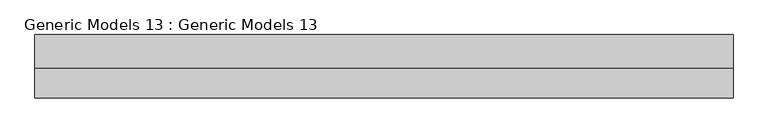
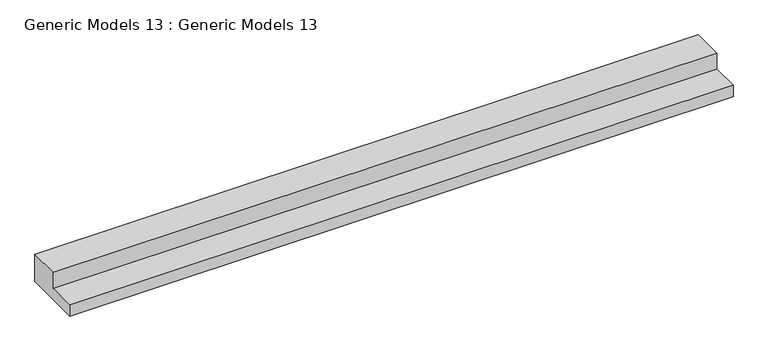
"""IFC4 building model written with IfcOpenShell, lengths in millimetres: proxy geometry, Generic Models 13 : Generic Models 13."""

from ifc_helpers import new_model, si_unit, frame, origin, place, context, project, spatial, polyline, outline, extrude, source, transform, mapped, element, save


def generic_models_13_generic_models_13_4f71b6b5(model_context):
    return source(origin(), model_context, "Body", "SweptSolid", [
        extrude(outline(polyline([(-11867.7407184, 0.0), (-12502.7407184, 0.0), (-12502.7407184, 127.0), (-12204.0599422, 127.0), (-12204.0599422, 304.8), (-11867.7407184, 304.8), (-11867.7407184, 0.0)])), frame((-7911.9236584, 0.0, 0.0), z_axis=(1.0, 0.0, 0.0), x_axis=(0.0, 1.0, 0.0)), (0.0, 0.0, 1.0), 6992.7053576),
    ])


if __name__ == "__main__":
    model = new_model("IFC4")
    model_context = context("Model", 3, world=origin())
    ifc_project = project(units=[si_unit("LENGTHUNIT", "METRE", prefix="MILLI")], contexts=[model_context])
    site = spatial("IfcSite", under=ifc_project)
    building = spatial("IfcBuilding", under=site)
    placement = place(None, origin())
    generic_models_13_generic_models_13_shape = generic_models_13_generic_models_13_4f71b6b5(model_context)
    element("IfcBuildingElementProxy", 1, Name="Generic Models 13 : Generic Models 13", ObjectType="Generic Models 13 : Generic Models 13", at=placement, inside=building, context=model_context, shape_type="MappedRepresentation", body=[
        mapped(generic_models_13_generic_models_13_shape, transform((0.0, 0.0, 0.0), x_axis=(1.0, 0.0, 0.0), y_axis=(0.0, 1.0, 0.0), z_axis=(0.0, 0.0, 1.0))),
    ])
    save(model, "model.ifc")

# Revit data of these elements
# Element 1 (IfcBuildingElementProxy, "Generic Models 13 : Generic Models 13")
#   Materials on its faces: "Concrete, Cast-in-Place gray"
# Materials
#   "Concrete, Cast-in-Place gray": class "Concrete", colour RGB 192 192 192, transparency 0, Description = "Cast-in-place concrete", Cost = 0
